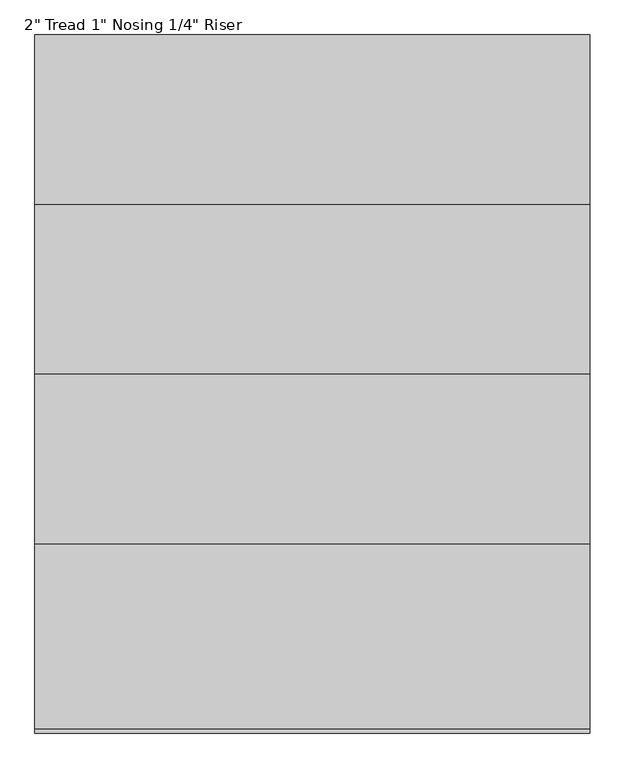
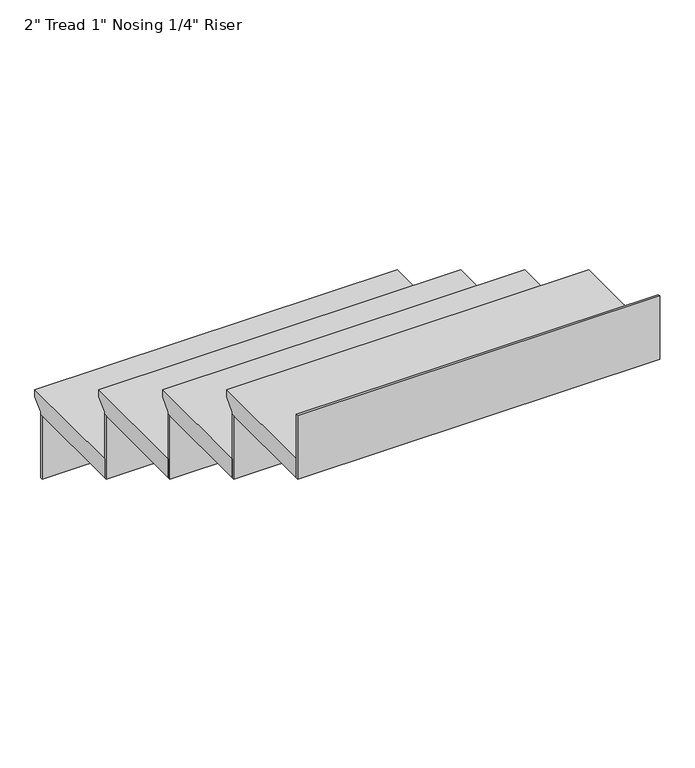
"""IFC4 building model written with IfcOpenShell, lengths in millimetres: stair flight geometry."""

from ifc_helpers import new_model, si_unit, frame, origin, place, context, project, spatial, polyline, outline, extrude, source, transform, mapped, element, save


def stair_flight_fe606327(model_context):
    return source(origin(), model_context, "Body", "SweptSolid", [
        extrude(outline(polyline([(22889.9216096, 42845.2839133), (23194.7216096, 42845.2839133), (23194.7216096, 42826.2339133), (23169.3216096, 42800.8339133), (23169.3216096, 42794.4839133), (22889.9216096, 42794.4839133), (22889.9216096, 42845.2839133)])), frame((-2398.2415084, 0.0, 0.0), z_axis=(1.0, 0.0, 0.0), x_axis=(0.0, 1.0, 0.0)), (0.0, 0.0, 1.0), 914.4),
        extrude(outline(polyline([(-2398.2415084, 23162.9716096), (-2398.2415084, 23169.3216096), (-1483.8415084, 23169.3216096), (-1483.8415084, 23162.9716096), (-2398.2415084, 23162.9716096)])), frame((0.0, 0.0, 42625.1505799), z_axis=(0.0, 0.0, 1.0), x_axis=(1.0, 0.0, 0.0)), (0.0, 0.0, 1.0), 169.3333333),
        extrude(outline(polyline([(-2398.2415084, 22883.5716096), (-2398.2415084, 22889.9216096), (-1483.8415084, 22889.9216096), (-1483.8415084, 22883.5716096), (-2398.2415084, 22883.5716096)])), frame((0.0, 0.0, 42794.4839133), z_axis=(0.0, 0.0, 1.0), x_axis=(1.0, 0.0, 0.0)), (0.0, 0.0, 1.0), 169.3333333),
        extrude(outline(polyline([(22610.5216096, 43014.6172466), (22915.3216096, 43014.6172466), (22915.3216096, 42995.5672466), (22889.9216096, 42970.1672466), (22889.9216096, 42963.8172466), (22610.5216096, 42963.8172466), (22610.5216096, 43014.6172466)])), frame((-2398.2415084, 0.0, 0.0), z_axis=(1.0, 0.0, 0.0), x_axis=(0.0, 1.0, 0.0)), (0.0, 0.0, 1.0), 914.4),
        extrude(outline(polyline([(-2398.2415084, 22604.1716096), (-2398.2415084, 22610.5216096), (-1483.8415084, 22610.5216096), (-1483.8415084, 22604.1716096), (-2398.2415084, 22604.1716096)])), frame((0.0, 0.0, 42963.8172466), z_axis=(0.0, 0.0, 1.0), x_axis=(1.0, 0.0, 0.0)), (0.0, 0.0, 1.0), 169.3333333),
        extrude(outline(polyline([(22331.1216096, 43183.9505799), (22635.9216096, 43183.9505799), (22635.9216096, 43164.9005799), (22610.5216096, 43139.5005799), (22610.5216096, 43133.1505799), (22331.1216096, 43133.1505799), (22331.1216096, 43183.9505799)])), frame((-2398.2415084, 0.0, 0.0), z_axis=(1.0, 0.0, 0.0), x_axis=(0.0, 1.0, 0.0)), (0.0, 0.0, 1.0), 914.4),
        extrude(outline(polyline([(-2398.2415084, 22324.7716096), (-2398.2415084, 22331.1216096), (-1483.8415084, 22331.1216096), (-1483.8415084, 22324.7716096), (-2398.2415084, 22324.7716096)])), frame((0.0, 0.0, 43133.1505799), z_axis=(0.0, 0.0, 1.0), x_axis=(1.0, 0.0, 0.0)), (0.0, 0.0, 1.0), 169.3333333),
        extrude(outline(polyline([(-2398.2415084, 22045.3716096), (-2398.2415084, 22051.7216096), (-1483.8415084, 22051.7216096), (-1483.8415084, 22045.3716096), (-2398.2415084, 22045.3716096)])), frame((0.0, 0.0, 43302.4839133), z_axis=(0.0, 0.0, 1.0), x_axis=(1.0, 0.0, 0.0)), (0.0, 0.0, 1.0), 169.3333333),
        extrude(outline(polyline([(22051.7216096, 43353.2839133), (22356.5216096, 43353.2839133), (22356.5216096, 43334.2339133), (22331.1216096, 43308.8339133), (22331.1216096, 43302.4839133), (22051.7216096, 43302.4839133), (22051.7216096, 43353.2839133)])), frame((-2398.2415084, 0.0, 0.0), z_axis=(1.0, 0.0, 0.0), x_axis=(0.0, 1.0, 0.0)), (0.0, 0.0, 1.0), 914.4),
    ])


if __name__ == "__main__":
    model = new_model("IFC4")
    model_context = context("Model", 3, world=origin())
    ifc_project = project(units=[si_unit("LENGTHUNIT", "METRE", prefix="MILLI")], contexts=[model_context])
    site = spatial("IfcSite", under=ifc_project)
    building = spatial("IfcBuilding", under=site)
    placement = place(None, origin())
    stair_flight_shape = stair_flight_fe606327(model_context)
    element("IfcStairFlight", 1, ObjectType="2\" Tread 1\" Nosing 1/4\" Riser", at=placement, inside=building, context=model_context, shape_type="MappedRepresentation", body=[
        mapped(stair_flight_shape, transform((0.0, 0.0, 0.0), x_axis=(1.0, 0.0, 0.0), y_axis=(0.0, 1.0, 0.0), z_axis=(0.0, 0.0, 1.0))),
    ])
    save(model, "model.ifc")
